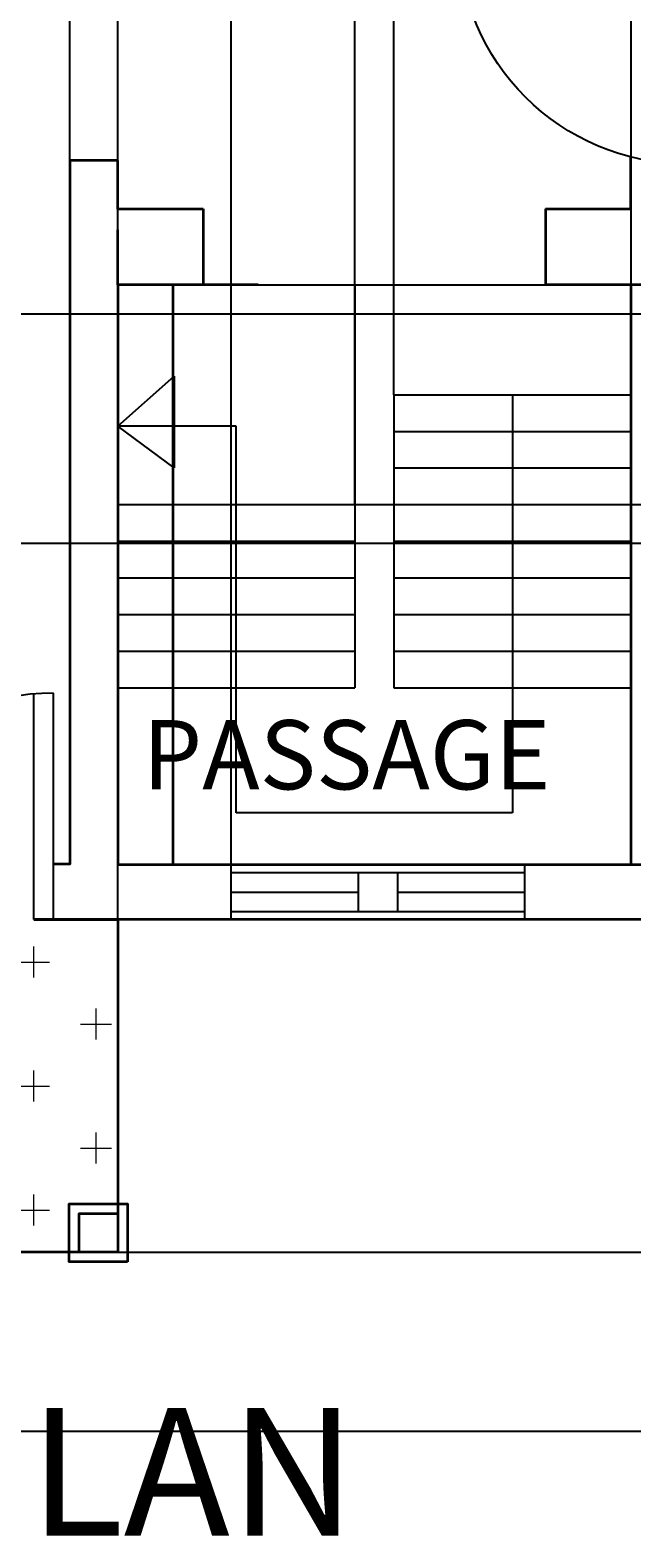
# Model space of a CAD drawing. Units: millimetres. Extents: x 19292 to 100733, y 12374 to 26974.
# Tile 15 of 24: x 31036 to 33498, y 12374 to 18550. Entities that reach past the tile are written whole.
import ezdxf

# ---------------------------------------------------------------- set-up
doc = ezdxf.new("R2010")
doc.units = ezdxf.units.MM
for name, color, linetype, lineweight in [('A-ANNO-DIMS', 2, 'Continuous', 18), ('A-ANNO-TEXT', 7, 'Continuous', 35), ('A-AREA-IDEN', 3, 'Continuous', 25), ('A-DOOR', 4, 'Continuous', 25), ('A-FLOR-PATT', 252, 'Continuous', 13), ('A-FLOR-STRS', 1, 'Continuous', 25), ('A-GLAZ', 3, 'Continuous', 25), ('A-WALL', 7, 'Continuous', 35)]:
    doc.layers.add(name, color=color, linetype=linetype, lineweight=lineweight)
doc.layers.add('WINDOWS', color=50, linetype='Continuous')
doc.styles.get("Standard").update_dxf_attribs({"font": 'arial.ttf'})
doc.dimstyles.get("Standard").update_dxf_attribs({"dimtxt": 0.18, "dimasz": 0.18, "dimexe": 0.18, "dimexo": 0.0625, "dimgap": 0.09, "dimtad": 0, "dimtih": 1, "dimtoh": 1, "dimdec": 4, "dimzin": 0, "dimdsep": 46, "dimtxsty": 'Standard', "dimcen": 0.09, "dimadec": 0, "dimazin": 0, "dimtfac": 1, "dimtdec": 4, "dimtofl": 0, "dimtmove": 0, "dimatfit": 3, "dimfxl": 1, "dimtolj": 1, "dimtzin": 0, "dimarcsym": 0})

# ---------------------------------------------------------------- blocks, each defined once
blk = doc.blocks.new('WW')
at = {"layer": 'WINDOWS'}
for p, q in [((-5183.9, -4940.9), (-3983.9, -4940.9)), ((-4663.9, -4940.9), (-4663.9, -5100.9)), ((-4503.9, -4940.9), (-4503.9, -5100.9)), ((-4503.9, -4940.9), (-4503.9, -5100.9)), ((-5183.9, -5020.9), (-4663.9, -5020.9)), ((-4503.9, -5020.9), (-3983.9, -5020.9)), ((-5183.9, -5100.9), (-3983.9, -5100.9))]:
    blk.add_line(p, q, dxfattribs=at)
for points in [[(-5183.9, -5133.4), (-5183.9, -4908.4)], [(-3983.9, -4908.4), (-3983.9, -5133.4)]]:
    blk.add_lwpolyline(points, dxfattribs=at)
blk = doc.blocks.new('DOOR-900')
for p, q in [((927.7, 80), (0, 80)), ((927.7, 0), (927.7, 80)), ((927.7, 0), (927.7, 80)), ((927.7, 0), (0, 0))]:
    blk.add_line(p, q)
blk.add_arc((927.7, 0), 927.7, 90, 180)
blk = doc.blocks.new('*D70')
at = {"layer": 'A-ANNO-DIMS', "color": 0, "lineweight": -2, "transparency": 16777216}
for p, q in [((23573.9, 17387.7), (36879.3, 17387.7)), ((36879.2, 17387.6), (36879.2, 16917.9)), ((36879.2, 16447.9), (36879.2, 16917.6)), ((23573.9, 16447.7), (36879.3, 16447.7))]:
    blk.add_line(p, q, dxfattribs=at)
at = {"layer": 'A-ANNO-DIMS', "color": 0, "transparency": 16777216}
for points in [[(36879.1, 17387.6), (36879.2, 17387.6), (36879.2, 17387.7)], [(36879.1, 16447.9), (36879.2, 16447.9), (36879.2, 16447.7)]]:
    blk.add_solid(points, dxfattribs=at)
at = {"layer": 'Defpoints', "color": 0, "transparency": 16777216}
for p in [(23573.8, 17387.7), (36879.2, 17387.7), (23573.8, 16447.7)]:
    blk.add_point(p, dxfattribs=at)
at = {"layer": 'A-ANNO-DIMS', "color": 0, "transparency": 16777216, "insert": (36879.2, 16917.7), "char_height": 0.18, "attachment_point": 5}
blk.add_mtext('\\A1;940', dxfattribs=at)
blk = doc.blocks.new('*D72')
at = {"layer": 'A-ANNO-DIMS', "color": 0, "lineweight": -2, "transparency": 16777216}
for p, q in [((33719.9, 14906.4), (36879.3, 14906.4)), ((36879.2, 14906.2), (36879.2, 14225.4)), ((36879.2, 13544.2), (36879.2, 14225)), ((31394.9, 13544), (36879.3, 13544))]:
    blk.add_line(p, q, dxfattribs=at)
at = {"layer": 'A-ANNO-DIMS', "color": 0, "transparency": 16777216}
for points in [[(36879.1, 14906.2), (36879.2, 14906.2), (36879.2, 14906.4)], [(36879.1, 13544.2), (36879.2, 13544.2), (36879.2, 13544)]]:
    blk.add_solid(points, dxfattribs=at)
at = {"layer": 'Defpoints', "color": 0, "transparency": 16777216}
for p in [(33719.8, 14906.4), (36879.2, 14906.4), (31394.8, 13544)]:
    blk.add_point(p, dxfattribs=at)
at = {"layer": 'A-ANNO-DIMS', "color": 0, "transparency": 16777216, "insert": (36879.2, 14225.2), "char_height": 0.18, "attachment_point": 5}
blk.add_mtext('\\A1;1362.4', dxfattribs=at)
blk = doc.blocks.new('*D79')
at = {"layer": 'A-ANNO-DIMS', "color": 0, "lineweight": -2, "transparency": 16777216}
for p, q in [((22694.1, 22860.7), (22694.1, 12808.8)), ((36144.2, 15985.7), (36144.2, 12808.8)), ((22694.3, 12809), (29418.7, 12809)), ((36144, 12809), (29419.6, 12809))]:
    blk.add_line(p, q, dxfattribs=at)
at = {"layer": 'A-ANNO-DIMS', "color": 0, "transparency": 16777216}
for points in [[(22694.3, 12809), (22694.3, 12809), (22694.1, 12809)], [(36144, 12809), (36144, 12809), (36144.2, 12809)]]:
    blk.add_solid(points, dxfattribs=at)
at = {"layer": 'Defpoints', "color": 0, "transparency": 16777216}
for p in [(22694.1, 22860.7), (36144.2, 15985.7), (36144.2, 12809)]:
    blk.add_point(p, dxfattribs=at)
at = {"layer": 'A-ANNO-DIMS', "color": 0, "transparency": 16777216, "insert": (29419.2, 12809), "char_height": 0.18, "attachment_point": 5}
blk.add_mtext('\\A1;13450', dxfattribs=at)
blk = doc.blocks.new('*D82')
at = {"layer": 'A-ANNO-DIMS', "color": 0, "lineweight": -2, "transparency": 16777216}
for p, q in [((27198.8, 13562.8), (27198.8, 23555.9)), ((27199, 23555.7), (29296.4, 23555.7)), ((31394.6, 23555.7), (29297.2, 23555.7)), ((31394.8, 13544.1), (31394.8, 23555.9))]:
    blk.add_line(p, q, dxfattribs=at)
at = {"layer": 'A-ANNO-DIMS', "color": 0, "transparency": 16777216}
for points in [[(27199, 23555.8), (27199, 23555.7), (27198.8, 23555.7)], [(31394.6, 23555.8), (31394.6, 23555.7), (31394.8, 23555.7)]]:
    blk.add_solid(points, dxfattribs=at)
at = {"layer": 'Defpoints', "color": 0, "transparency": 16777216}
for p in [(31394.8, 23555.7), (27198.8, 13562.7), (31394.8, 13544)]:
    blk.add_point(p, dxfattribs=at)
at = {"layer": 'A-ANNO-DIMS', "color": 0, "transparency": 16777216, "insert": (29296.8, 23555.7), "char_height": 0.18, "attachment_point": 5}
blk.add_mtext('\\A1;4196', dxfattribs=at)
blk = doc.blocks.new('*D83')
at = {"layer": 'A-ANNO-DIMS', "color": 0, "lineweight": -2, "transparency": 16777216}
for p, q in [((31394.8, 15131.5), (31394.8, 23555.9)), ((31395, 23555.7), (31626.3, 23555.7)), ((31858.6, 23555.7), (31627.2, 23555.7)), ((31858.7, 15131.5), (31858.7, 23555.9))]:
    blk.add_line(p, q, dxfattribs=at)
at = {"layer": 'A-ANNO-DIMS', "color": 0, "transparency": 16777216}
for points in [[(31395, 23555.8), (31395, 23555.7), (31394.8, 23555.7)], [(31858.6, 23555.8), (31858.6, 23555.7), (31858.7, 23555.7)]]:
    blk.add_solid(points, dxfattribs=at)
at = {"layer": 'Defpoints', "color": 0, "transparency": 16777216}
for p in [(31858.7, 23555.7), (31394.8, 15131.4), (31858.7, 15131.4)]:
    blk.add_point(p, dxfattribs=at)
at = {"layer": 'A-ANNO-DIMS', "color": 0, "transparency": 16777216, "insert": (31626.8, 23555.7), "char_height": 0.18, "attachment_point": 5}
blk.add_mtext('\\A1;463.95', dxfattribs=at)
blk = doc.blocks.new('*D86')
at = {"layer": 'A-ANNO-DIMS', "color": 0, "lineweight": -2, "transparency": 16777216}
for p, q in [((27198.8, 15132.8), (27198.8, 23555.9)), ((27199, 23555.7), (29198.5, 23555.7)), ((31198.6, 23555.7), (29199.2, 23555.7)), ((31198.8, 15132.8), (31198.8, 23555.9))]:
    blk.add_line(p, q, dxfattribs=at)
at = {"layer": 'A-ANNO-DIMS', "color": 0, "transparency": 16777216}
for points in [[(27199, 23555.8), (27199, 23555.7), (27198.8, 23555.7)], [(31198.6, 23555.8), (31198.6, 23555.7), (31198.8, 23555.7)]]:
    blk.add_solid(points, dxfattribs=at)
at = {"layer": 'Defpoints', "color": 0, "transparency": 16777216}
for p in [(31198.8, 23555.7), (27198.8, 15132.7), (31198.8, 15132.7)]:
    blk.add_point(p, dxfattribs=at)
at = {"layer": 'A-ANNO-DIMS', "color": 0, "transparency": 16777216, "insert": (29198.8, 23555.7), "char_height": 0.18, "attachment_point": 5}
blk.add_mtext('\\A1;4000', dxfattribs=at)
blk = doc.blocks.new('*D87')
at = {"layer": 'A-ANNO-DIMS', "color": 0, "lineweight": -2, "transparency": 16777216}
for p, q in [((32524.8, 17056.5), (32524.8, 23555.9)), ((32525, 23555.7), (33009.5, 23555.7)), ((33494.6, 23555.7), (33010.1, 23555.7)), ((33494.8, 17056.5), (33494.8, 23555.9))]:
    blk.add_line(p, q, dxfattribs=at)
at = {"layer": 'A-ANNO-DIMS', "color": 0, "transparency": 16777216}
for points in [[(32525, 23555.8), (32525, 23555.7), (32524.8, 23555.7)], [(33494.6, 23555.8), (33494.6, 23555.7), (33494.8, 23555.7)]]:
    blk.add_solid(points, dxfattribs=at)
at = {"layer": 'Defpoints', "color": 0, "transparency": 16777216}
for p in [(33494.8, 23555.7), (32524.8, 17056.4), (33494.8, 17056.4)]:
    blk.add_point(p, dxfattribs=at)
at = {"layer": 'A-ANNO-DIMS', "color": 0, "transparency": 16777216, "insert": (33009.8, 23555.7), "char_height": 0.18, "attachment_point": 5}
blk.add_mtext('\\A1;970', dxfattribs=at)
blk = doc.blocks.new('*D88')
at = {"layer": 'A-ANNO-DIMS', "color": 0, "lineweight": -2, "transparency": 16777216}
for p, q in [((31394.8, 16606.5), (31394.8, 23555.9)), ((31395, 23555.7), (31879.5, 23555.7)), ((32364.6, 23555.7), (31880.1, 23555.7)), ((32364.8, 16606.5), (32364.8, 23555.9))]:
    blk.add_line(p, q, dxfattribs=at)
at = {"layer": 'A-ANNO-DIMS', "color": 0, "transparency": 16777216}
for points in [[(31395, 23555.8), (31395, 23555.7), (31394.8, 23555.7)], [(32364.6, 23555.8), (32364.6, 23555.7), (32364.8, 23555.7)]]:
    blk.add_solid(points, dxfattribs=at)
at = {"layer": 'Defpoints', "color": 0, "transparency": 16777216}
for p in [(32364.8, 23555.7), (31394.8, 16606.4), (32364.8, 16606.4)]:
    blk.add_point(p, dxfattribs=at)
at = {"layer": 'A-ANNO-DIMS', "color": 0, "transparency": 16777216, "insert": (31879.8, 23555.7), "char_height": 0.18, "attachment_point": 5}
blk.add_mtext('\\A1;970', dxfattribs=at)
blk = doc.blocks.new('*D89')
at = {"layer": 'A-ANNO-DIMS', "color": 0, "lineweight": -2, "transparency": 16777216}
for p, q in [((31394.9, 17506.4), (36879.3, 17506.4)), ((36879.2, 17506.2), (36879.2, 17056.6)), ((36879.2, 16606.6), (36879.2, 17056.2)), ((31394.9, 16606.4), (36879.3, 16606.4))]:
    blk.add_line(p, q, dxfattribs=at)
at = {"layer": 'A-ANNO-DIMS', "color": 0, "transparency": 16777216}
for points in [[(36879.1, 17506.2), (36879.2, 17506.2), (36879.2, 17506.4)], [(36879.1, 16606.6), (36879.2, 16606.6), (36879.2, 16606.4)]]:
    blk.add_solid(points, dxfattribs=at)
at = {"layer": 'Defpoints', "color": 0, "transparency": 16777216}
for p in [(31394.8, 17506.4), (31394.8, 16606.4), (36879.2, 16606.4)]:
    blk.add_point(p, dxfattribs=at)
at = {"layer": 'A-ANNO-DIMS', "color": 0, "transparency": 16777216, "insert": (36879.2, 17056.4), "char_height": 0.18, "attachment_point": 5}
blk.add_mtext('\\A1;900', dxfattribs=at)

msp = doc.modelspace()

# ---------------------------------------------------------------- hatches: boundary and pattern name
at = {"layer": 'A-FLOR-PATT'}
h = msp.add_hatch(dxfattribs=at)
h.set_pattern_fill('CROSS', color=256, scale=40)
h.paths.add_polyline_path([(36144.169, 19010.725), (33719.169, 19010.725), (33719.169, 18850.725), (33719.169, 18003.026), (33719.169, 15985.725), (36144.169, 15985.725)])
h.paths.add_polyline_path([(36144.132, 22460.725), (34419.132, 22460.725), (34419.132, 22208.026, -0.34415073), (35121.831, 21308.026), (34419.132, 21308.026), (34419.132, 21260.725), (36144.132, 21260.725)])
h.paths.add_polyline_path([(34419.132, 22208.026), (34419.132, 21388.026), (35118.375, 21388.026, 0.32018294)], flags=17)
h.paths.add_polyline_path([(31169.132, 22460.725), (28369.132, 22460.725), (28369.132, 21460.725), (31169.132, 21460.725)])
h.paths.add_polyline_path([(34010.406, 17316.149), (36018.156, 17316.149), (36018.156, 17722.778), (34010.406, 17722.778)], flags=24)
h.paths.add_polyline_path([(34456.896, 21920.301), (35605.434, 21920.301), (35605.434, 22313.518), (34456.896, 22313.518)], flags=25)
h.paths.add_polyline_path([(29263.068, 21823.707), (30421.489, 21823.707), (30421.489, 22034.008), (29263.068, 22034.008)], flags=24)
h = msp.add_hatch(dxfattribs=at)
h.set_pattern_fill('CROSS', color=256, scale=40)
h.paths.add_polyline_path([(31394.799, 14906.403), (31051.542, 14906.403), (29468.571, 14906.403), (27198.815, 14906.403), (27198.815, 13543.993), (31394.799, 13543.993)])
h.paths.add_polyline_path([(27828.096, 14036.581), (30629.164, 14036.581), (30629.164, 14443.478), (27828.096, 14443.478)], flags=24)

# ---------------------------------------------------------------- linework, layer by layer
at = {"layer": 'A-DOOR'}
for p, q in [((31051.542, 14906.403), (31051.542, 15834.102)), ((31131.542, 14906.403), (31131.542, 15834.102)), ((31131.542, 14906.403), (31051.542, 14906.403)), ((31131.542, 14906.403), (31051.542, 14906.403))]:
    msp.add_line(p, q, dxfattribs=at)
msp.add_arc((31131.542, 14906.403), 927.699, 90, 180, dxfattribs=at)
at = {"layer": 'A-FLOR-STRS'}
for p, q in [((31394.799, 17506.403), (32364.799, 17506.403)), ((32364.799, 17506.403), (32364.799, 15856.403)), ((31394.799, 16927.763), (31625.322, 17131.846)), ((31625.322, 17131.846), (31625.322, 16756.403)), ((32524.799, 17056.403), (33494.799, 17056.403)), ((32524.799, 17056.403), (32524.799, 15856.403)), ((33009.799, 17056.403), (33009.799, 15343.431)), ((31879.799, 16927.763), (31394.799, 16927.763)), ((31625.322, 16756.403), (31394.799, 16927.763)), ((31879.799, 15343.431), (31879.799, 16927.763)), ((32524.799, 16906.403), (33494.799, 16906.403)), ((32524.799, 16756.403), (33494.799, 16756.403)), ((31394.799, 16606.403), (32364.799, 16606.403)), ((32524.799, 16606.403), (33494.799, 16606.403)), ((31394.799, 16456.403), (32364.799, 16456.403)), ((32524.799, 16456.403), (33494.799, 16456.403)), ((31394.799, 16306.403), (32364.799, 16306.403)), ((32524.799, 16306.403), (33494.799, 16306.403)), ((31394.799, 16156.403), (32364.799, 16156.403)), ((32524.799, 16156.403), (33494.799, 16156.403)), ((31394.799, 16006.403), (32364.799, 16006.403)), ((32524.799, 16006.403), (33494.799, 16006.403)), ((31394.799, 15856.403), (32364.799, 15856.403)), ((32524.799, 15856.403), (33494.799, 15856.403)), ((33009.799, 15343.431), (31879.799, 15343.431))]:
    msp.add_line(p, q, dxfattribs=at)
at = {"layer": 'A-WALL'}
for p, q in [((31394.132, 18015.368), (31198.815, 18015.368)), ((31744.132, 17817.987), (31744.132, 17506.403)), ((33144.132, 17817.987), (33144.132, 17506.403)), ((31394.799, 17506.403), (31394.799, 17731.403))]:
    msp.add_line(p, q, dxfattribs=at)
for points in [[(31198.815, 18015.368), (31198.815, 15132.748), (31131.542, 15132.748)], [(31394.132, 18015.368), (31394.132, 17817.987), (31744.132, 17817.987)], [(33144.132, 17817.987), (33494.132, 17817.987), (33494.132, 18030.734)], [(31744.132, 17506.403), (31394.799, 17506.403), (31394.799, 15131.403), (33494.799, 15131.403), (33494.799, 17506.403), (33144.132, 17506.403)], [(31969.132, 17506.403), (31619.799, 17506.403), (31619.799, 15131.403), (33719.799, 15131.403), (33719.799, 17506.403), (33369.132, 17506.403)], [(33719.66, 15985.725), (33719.835, 14906.403), (31051.542, 14906.403)], [(31051.542, 14906.403), (31394.799, 14906.403), (31394.799, 13543.993), (27198.815, 13543.993), (27198.815, 14906.403), (29548.571, 14906.403)]]:
    msp.add_lwpolyline(points, dxfattribs=at)
for points in [[(31434.799, 13503.993), (31196.347, 13503.993), (31196.347, 13742.444), (31434.799, 13742.444)], [(31394.799, 13543.993), (31236.347, 13543.993), (31236.347, 13702.444), (31394.799, 13702.444)]]:
    msp.add_lwpolyline(points, close=True, dxfattribs=at)

# ---------------------------------------------------------------- block references
at = {"layer": 'A-DOOR', "extrusion": (0, 0, -1), "zscale": -1, "rotation": 180}
msp.add_blockref('DOOR-900', (-32791.471, 18930.725), dxfattribs=at)
at = {"layer": 'A-GLAZ'}
msp.add_blockref('WW', (37042.613, 20039.78), dxfattribs=at)

# ---------------------------------------------------------------- texts
at = {"layer": 'A-ANNO-TEXT'}
msp.add_text('GROUND FLOOR PLAN', height=523.26848, dxfattribs=at).set_placement((24968.619, 12383.031))
at = {"layer": 'A-AREA-IDEN'}
msp.add_text('PASSAGE', height=283.3894, dxfattribs=at).set_placement((31495.482, 15439.908))

# ---------------------------------------------------------------- dimensions: what is measured, and where the dimension line sits
at = {"layer": 'A-ANNO-DIMS'}
for base, p1, p2, override, picture, middle in [((31394.799, 23555.725), (27198.815, 13562.748), (31394.799, 13543.993), {"dimdec": 0, "dimlfac": 1, "dimrnd": 0, "dimzin": 0, "dimdsep": 46, "dimlunit": 2}, '*D82', (29296.807, 23555.725)), ((31198.815, 23555.725), (27198.815, 15132.748), (31198.815, 15132.748), {"dimdec": 0, "dimlfac": 1, "dimrnd": 0, "dimzin": 0, "dimdsep": 46, "dimlunit": 2}, '*D86', (29198.815, 23555.725)), ((31858.745, 23555.725), (31394.799, 15131.403), (31858.745, 15131.403), {"dimdec": 2, "dimlfac": 1, "dimrnd": 0, "dimzin": 0, "dimdsep": 46, "dimlunit": 2}, '*D83', (31626.772, 23555.725)), ((32364.799, 23555.725), (31394.799, 16606.403), (32364.799, 16606.403), {"dimdec": 0, "dimlfac": 1, "dimrnd": 0, "dimzin": 0, "dimdsep": 46, "dimlunit": 2}, '*D88', (31879.799, 23555.725)), ((33494.799, 23555.725), (32524.799, 17056.403), (33494.799, 17056.403), {"dimdec": 0, "dimlfac": 1, "dimrnd": 0, "dimzin": 0, "dimdsep": 46, "dimlunit": 2}, '*D87', (33009.799, 23555.725)), ((36144.169, 12808.993), (22694.132, 22860.725), (36144.169, 15985.725), {"dimdec": 0, "dimlfac": 1, "dimrnd": 0, "dimzin": 0, "dimdsep": 46, "dimlunit": 2}, '*D79', (29419.151, 12808.993))]:
    dim = msp.add_linear_dim(base=base, p1=p1, p2=p2, dimstyle='Standard', override=override, dxfattribs=at)
    dim.commit()
    dim.dimension.update_dxf_attribs({"geometry": picture, "text_midpoint": middle})
for base, p1, p2, override, picture, middle in [((36879.169, 16606.403), (31394.799, 17506.403), (31394.799, 16606.403), {"dimdec": 0, "dimlfac": 1, "dimrnd": 0, "dimzin": 0, "dimdsep": 46, "dimlunit": 2}, '*D89', (36879.169, 17056.403)), ((36879.169, 17387.748), (23573.815, 16447.748), (23573.815, 17387.748), {"dimdec": 0, "dimlfac": 1, "dimrnd": 0, "dimzin": 0, "dimdsep": 46, "dimlunit": 2}, '*D70', (36879.169, 16917.748)), ((36879.169, 14906.403), (31394.799, 13543.993), (33719.835, 14906.403), {"dimdec": 1, "dimlfac": 1, "dimrnd": 0, "dimzin": 0, "dimdsep": 46, "dimlunit": 2}, '*D72', (36879.169, 14225.198))]:
    dim = msp.add_linear_dim(base=base, p1=p1, p2=p2, angle=90, dimstyle='Standard', override=override, dxfattribs=at)
    dim.commit()
    dim.dimension.update_dxf_attribs({"geometry": picture, "text_midpoint": middle})

doc.saveas('drawing.dxf')
